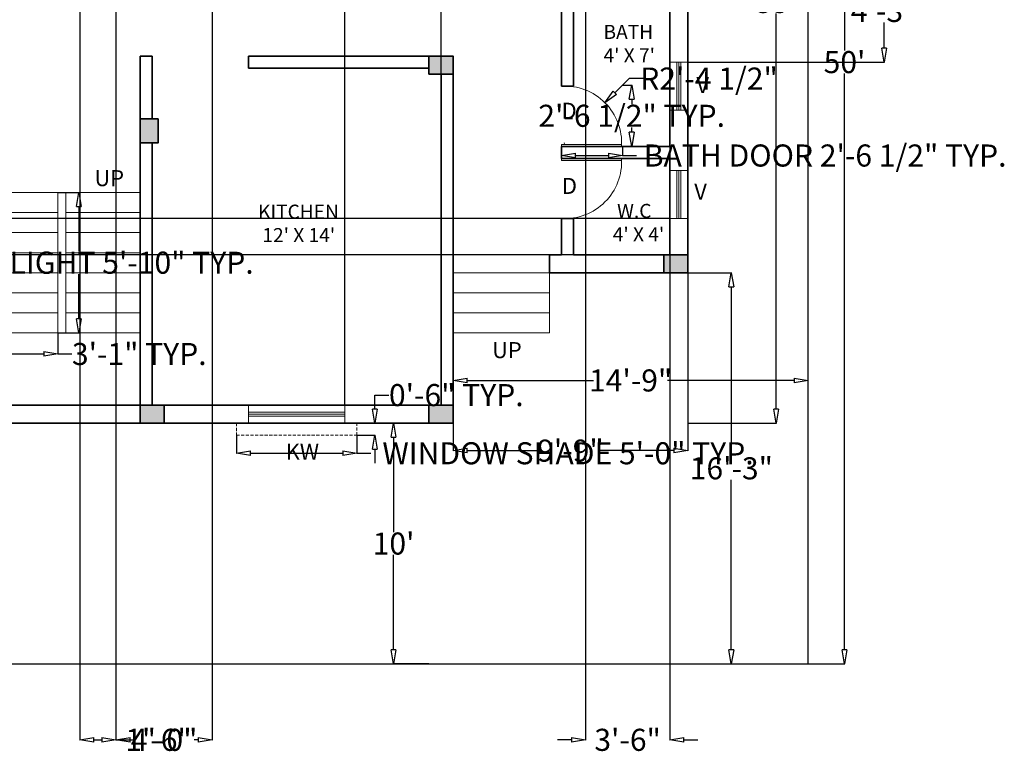
# Model space of a CAD drawing. Units: inches. Extents: x 668 to 1552, y 994 to 1684.
# Tile 3 of 4: x 1061 to 1552, y 994 to 1360. Entities that reach past the tile are written whole.
import ezdxf

# ---------------------------------------------------------------- set-up
doc = ezdxf.new("R2010")
doc.units = ezdxf.units.IN
doc.header["$LTSCALE"] = 2.5
doc.header["$MEASUREMENT"] = 0
doc.linetypes.add('HIDDEN', pattern=[0.375, 0.25, -0.125])
for name, color, linetype, lineweight, true_color in [('A-ANNO-DIMS', 175, 'Continuous', 13, 0x4554a5), ('A-ANNO-TEXT', 52, 'Continuous', 18, 0xc8c92d), ('A-DOOR', 152, 'Continuous', 18, 0x2776bb), ('A-FLOR-STRS', 165, 'Continuous', 18, 0x5e67af)]:
    doc.layers.add(name, color=color, linetype=linetype, lineweight=lineweight, true_color=true_color)
for name, color, linetype, lineweight in [('A-AREA-IDEN', 2, 'Continuous', 18), ('A-COLS', 7, 'Continuous', 35), ('A-COLS-PATT', 1, 'Continuous', 13), ('A-GLAZ', 4, 'Continuous', 18), ('A-WALL', 7, 'Continuous', 35), ('C-PROP', 1, 'Continuous', 25), ('sajjas', 210, 'HIDDEN', 13)]:
    doc.layers.add(name, color=color, linetype=linetype, lineweight=lineweight)
doc.styles.get("Standard").update_dxf_attribs({"font": 'arial.ttf'})
doc.dimstyles.get("Standard").update_dxf_attribs({"dimtxt": 11, "dimasz": 7, "dimexe": 0.18, "dimexo": 0.0625, "dimgap": 0.09, "dimtad": 0, "dimtih": 1, "dimtoh": 1, "dimdec": 0, "dimzin": 0, "dimdsep": 46, "dimlunit": 3, "dimtxsty": 'Standard', "dimblk": 'CLOSEDBLANK', "dimcen": 0.09, "dimadec": 0, "dimazin": 0, "dimtfac": 1, "dimtdec": 0, "dimtofl": 0, "dimtmove": 0, "dimatfit": 3, "dimldrblk": 'CLOSEDBLANK', "dimfxl": 1, "dimtolj": 1, "dimtzin": 0, "dimarcsym": 0})

# ---------------------------------------------------------------- blocks, each defined once
blk = doc.blocks.new('_ClosedBlank')
at = {"color": 0, "linetype": 'ByBlock', "lineweight": -2}
for p, q in [((-1, 0.167), (0, 0)), ((-1, 0.167), (-1, -0.167)), ((0, 0), (-1, -0.167))]:
    blk.add_line(p, q, dxfattribs=at)
blk = doc.blocks.new('*D2')
at = {"layer": 'A-ANNO-DIMS', "color": 0, "lineweight": -2, "ltscale": 2.5, "transparency": 16777216}
for p, q in [((1454.43, 1639.35), (1472.67, 1639.35)), ((1472.49, 1632.35), (1472.49, 1345.06)), ((1472.49, 1046.35), (1472.49, 1333.64)), ((1454.43, 1039.35), (1472.67, 1039.35))]:
    blk.add_line(p, q, dxfattribs=at)
at = {"layer": 'Defpoints', "color": 0, "ltscale": 2.5, "transparency": 16777216}
for p in [(1454.36, 1639.35), (1454.36, 1039.35), (1472.49, 1039.35)]:
    blk.add_point(p, dxfattribs=at)
at = {"layer": 'A-ANNO-DIMS', "color": 0, "lineweight": -2, "ltscale": 2.5, "transparency": 16777216, "xscale": 7, "yscale": 7, "zscale": 7}
for p, rotation in [((1472.49, 1639.35), 90), ((1472.49, 1039.35), 270)]:
    blk.add_blockref('_ClosedBlank', p, dxfattribs=dict(at, rotation=rotation))
at = {"layer": 'A-ANNO-DIMS', "color": 0, "ltscale": 2.5, "transparency": 16777216, "insert": (1472.49, 1339.35), "char_height": 11, "attachment_point": 5}
blk.add_mtext("\\A1;50'", dxfattribs=at)
blk = doc.blocks.new('*D9')
at = {"layer": 'A-ANNO-DIMS', "color": 0, "lineweight": -2, "ltscale": 2.5, "transparency": 16777216}
for p, q in [((1394.43, 1579.35), (1438.61, 1579.35)), ((1438.43, 1572.35), (1438.43, 1375.06)), ((1438.43, 1166.35), (1438.43, 1363.64)), ((1394.43, 1159.35), (1438.61, 1159.35))]:
    blk.add_line(p, q, dxfattribs=at)
at = {"layer": 'Defpoints', "color": 0, "ltscale": 2.5, "transparency": 16777216}
for p in [(1394.36, 1579.35), (1394.36, 1159.35), (1438.43, 1159.35)]:
    blk.add_point(p, dxfattribs=at)
at = {"layer": 'A-ANNO-DIMS', "color": 0, "lineweight": -2, "ltscale": 2.5, "transparency": 16777216, "xscale": 7, "yscale": 7, "zscale": 7}
for p, rotation in [((1438.43, 1579.35), 90), ((1438.43, 1159.35), 270)]:
    blk.add_blockref('_ClosedBlank', p, dxfattribs=dict(at, rotation=rotation))
at = {"layer": 'A-ANNO-DIMS', "color": 0, "ltscale": 2.5, "transparency": 16777216, "insert": (1438.43, 1369.35), "char_height": 11, "attachment_point": 5}
blk.add_mtext("\\A1;35'", dxfattribs=at)
blk = doc.blocks.new('*D10')
at = {"layer": 'A-ANNO-DIMS', "color": 0, "lineweight": -2, "ltscale": 2.5, "transparency": 16777216}
for p, q in [((1394.43, 1234.35), (1416.24, 1234.35)), ((1416.06, 1227.35), (1416.06, 1142.56)), ((1416.06, 1046.35), (1416.06, 1131.14)), ((1394.43, 1039.35), (1416.24, 1039.35))]:
    blk.add_line(p, q, dxfattribs=at)
at = {"layer": 'Defpoints', "color": 0, "ltscale": 2.5, "transparency": 16777216}
for p in [(1394.36, 1234.35), (1394.36, 1039.35), (1416.06, 1039.35)]:
    blk.add_point(p, dxfattribs=at)
at = {"layer": 'A-ANNO-DIMS', "color": 0, "lineweight": -2, "ltscale": 2.5, "transparency": 16777216, "xscale": 7, "yscale": 7, "zscale": 7}
for p, rotation in [((1416.06, 1234.35), 90), ((1416.06, 1039.35), 270)]:
    blk.add_blockref('_ClosedBlank', p, dxfattribs=dict(at, rotation=rotation))
at = {"layer": 'A-ANNO-DIMS', "color": 0, "ltscale": 2.5, "transparency": 16777216, "insert": (1416.06, 1136.85), "char_height": 11, "attachment_point": 5}
blk.add_mtext('\\A1;16\'-3"', dxfattribs=at)
blk = doc.blocks.new('*D11')
at = {"layer": 'A-ANNO-DIMS', "color": 0, "lineweight": -2, "ltscale": 2.5, "transparency": 16777216}
for p, q in [((1277.36, 1234.29), (1277.36, 1145.5)), ((1394.36, 1234.29), (1394.36, 1145.5)), ((1284.36, 1145.68), (1321.15, 1145.68)), ((1387.36, 1145.68), (1350.57, 1145.68))]:
    blk.add_line(p, q, dxfattribs=at)
at = {"layer": 'Defpoints', "color": 0, "ltscale": 2.5, "transparency": 16777216}
for p in [(1277.36, 1234.35), (1394.36, 1234.35), (1277.36, 1145.68)]:
    blk.add_point(p, dxfattribs=at)
at = {"layer": 'A-ANNO-DIMS', "color": 0, "lineweight": -2, "ltscale": 2.5, "transparency": 16777216, "xscale": 7, "yscale": 7, "zscale": 7, "rotation": 180}
blk.add_blockref('_ClosedBlank', (1277.36, 1145.68), dxfattribs=at)
at = {"layer": 'A-ANNO-DIMS', "color": 0, "lineweight": -2, "ltscale": 2.5, "transparency": 16777216, "xscale": 7, "yscale": 7, "zscale": 7}
blk.add_blockref('_ClosedBlank', (1394.36, 1145.68), dxfattribs=at)
at = {"layer": 'A-ANNO-DIMS', "color": 0, "ltscale": 2.5, "transparency": 16777216, "insert": (1335.86, 1145.68), "char_height": 11, "attachment_point": 5}
blk.add_mtext('\\A1;9\'-9"', dxfattribs=at)
blk = doc.blocks.new('*D12')
at = {"layer": 'A-ANNO-DIMS', "color": 0, "lineweight": -2, "ltscale": 2.5, "transparency": 16777216}
for p, q in [((1265.3, 1159.35), (1247.53, 1159.35)), ((1247.71, 1152.35), (1247.71, 1105.06)), ((1247.71, 1046.35), (1247.71, 1093.64)), ((1265.3, 1039.35), (1247.53, 1039.35))]:
    blk.add_line(p, q, dxfattribs=at)
at = {"layer": 'Defpoints', "color": 0, "ltscale": 2.5, "transparency": 16777216}
for p in [(1265.36, 1159.35), (1247.71, 1039.35), (1265.36, 1039.35)]:
    blk.add_point(p, dxfattribs=at)
at = {"layer": 'A-ANNO-DIMS', "color": 0, "lineweight": -2, "ltscale": 2.5, "transparency": 16777216, "xscale": 7, "yscale": 7, "zscale": 7}
for p, rotation in [((1247.71, 1159.35), 90), ((1247.71, 1039.35), 270)]:
    blk.add_blockref('_ClosedBlank', p, dxfattribs=dict(at, rotation=rotation))
at = {"layer": 'A-ANNO-DIMS', "color": 0, "ltscale": 2.5, "transparency": 16777216, "insert": (1247.71, 1099.35), "char_height": 11, "attachment_point": 5}
blk.add_mtext("\\A1;10'", dxfattribs=at)
blk = doc.blocks.new('*D13')
at = {"layer": 'A-ANNO-DIMS', "color": 0, "lineweight": -2, "ltscale": 2.5, "transparency": 16777216}
for p, q in [((1277.36, 1168.41), (1277.36, 1180.83)), ((1284.36, 1180.65), (1347.4, 1180.65)), ((1447.36, 1180.65), (1384.33, 1180.65)), ((1454.36, 1168.41), (1454.36, 1180.83))]:
    blk.add_line(p, q, dxfattribs=at)
at = {"layer": 'Defpoints', "color": 0, "ltscale": 2.5, "transparency": 16777216}
for p in [(1454.36, 1180.65), (1277.36, 1168.35), (1454.36, 1168.35)]:
    blk.add_point(p, dxfattribs=at)
at = {"layer": 'A-ANNO-DIMS', "color": 0, "lineweight": -2, "ltscale": 2.5, "transparency": 16777216, "xscale": 7, "yscale": 7, "zscale": 7, "rotation": 180}
blk.add_blockref('_ClosedBlank', (1277.36, 1180.65), dxfattribs=at)
at = {"layer": 'A-ANNO-DIMS', "color": 0, "lineweight": -2, "ltscale": 2.5, "transparency": 16777216, "xscale": 7, "yscale": 7, "zscale": 7}
blk.add_blockref('_ClosedBlank', (1454.36, 1180.65), dxfattribs=at)
at = {"layer": 'A-ANNO-DIMS', "color": 0, "ltscale": 2.5, "transparency": 16777216, "insert": (1365.86, 1180.65), "char_height": 11, "attachment_point": 5}
blk.add_mtext('\\A1;14\'-9"', dxfattribs=at)
blk = doc.blocks.new('WIN-48')
for p, q in [((0, 9), (48, 9)), ((0, 9), (0, 0)), ((48, 5.5), (0, 5.5)), ((48, 9), (48, 0)), ((48, 4.5), (0, 4.5)), ((48, 3.5), (0, 3.5)), ((0, 0), (48, 0))]:
    blk.add_line(p, q)
blk = doc.blocks.new('VENT-24')
for p, q in [((0, 9), (24, 9)), ((0, 0), (0, 9)), ((24, 5.5), (0.04, 5.5)), ((24, 9), (24, 0)), ((24, 0), (0, 0)), ((24, 4.5), (0.04, 4.5)), ((24, 3.5), (0.04, 3.5))]:
    blk.add_line(p, q)
blk = doc.blocks.new('SAJJA-60')
at = {"ltscale": 2.5}
blk.add_lwpolyline([(6, 6), (0, 6), (0, 0), (54, 0), (60, 0), (60, 6), (54, 6)], dxfattribs=at)
blk = doc.blocks.new('DOOR-BATH-30')
for p, q in [((0, 1), (30, 1)), ((0, 0), (30, 0))]:
    blk.add_line(p, q)
blk.add_arc((1.62, 1.62), 28.42, 356.7299, 93.2701)
blk = doc.blocks.new('STAIR-FLIGHT-37')
at = {"ltscale": 2.5}
for p, q in [((0, 70), (37, 70)), ((37, 0), (37, 70)), ((0, 60), (37, 60)), ((0, 50), (37, 50)), ((0, 40), (37, 40)), ((0, 30), (37, 30)), ((0, 20), (37, 20)), ((0, 10), (37, 10))]:
    blk.add_line(p, q, dxfattribs=at)
blk = doc.blocks.new('*D24')
at = {"layer": 'A-ANNO-DIMS', "color": 0, "lineweight": -2, "ltscale": 2.5, "transparency": 16777216}
for p, q in [((1169.36, 1153.29), (1169.36, 1144.17)), ((1229.36, 1153.29), (1229.36, 1144.17)), ((1176.36, 1144.35), (1222.36, 1144.35)), ((1229.36, 1144.35), (1236.36, 1144.35))]:
    blk.add_line(p, q, dxfattribs=at)
at = {"layer": 'Defpoints', "color": 0, "ltscale": 2.5, "transparency": 16777216}
for p in [(1169.36, 1153.35), (1229.36, 1153.35), (1229.36, 1144.35)]:
    blk.add_point(p, dxfattribs=at)
at = {"layer": 'A-ANNO-DIMS', "color": 0, "lineweight": -2, "ltscale": 2.5, "transparency": 16777216, "xscale": 7, "yscale": 7, "zscale": 7, "rotation": 180}
blk.add_blockref('_ClosedBlank', (1169.36, 1144.35), dxfattribs=at)
at = {"layer": 'A-ANNO-DIMS', "color": 0, "lineweight": -2, "ltscale": 2.5, "transparency": 16777216, "xscale": 7, "yscale": 7, "zscale": 7}
blk.add_blockref('_ClosedBlank', (1229.36, 1144.35), dxfattribs=at)
at = {"layer": 'A-ANNO-DIMS', "color": 0, "ltscale": 2.5, "transparency": 16777216, "insert": (1334.66, 1144.35), "char_height": 11, "attachment_point": 5}
blk.add_mtext('\\A1;WINDOW SHADE 5\'-0" TYP.', dxfattribs=at)
blk = doc.blocks.new('*D25')
at = {"layer": 'A-ANNO-DIMS', "color": 0, "lineweight": -2, "ltscale": 2.5, "transparency": 16777216}
for p, q in [((1238.36, 1166.35), (1238.36, 1173.35)), ((1238.36, 1173.35), (1245.36, 1173.35)), ((1229.43, 1159.35), (1238.54, 1159.35)), ((1229.43, 1153.35), (1238.54, 1153.35)), ((1238.36, 1146.35), (1238.36, 1139.35))]:
    blk.add_line(p, q, dxfattribs=at)
at = {"layer": 'Defpoints', "color": 0, "ltscale": 2.5, "transparency": 16777216}
for p in [(1229.36, 1159.35), (1238.36, 1159.35), (1229.36, 1153.35)]:
    blk.add_point(p, dxfattribs=at)
at = {"layer": 'A-ANNO-DIMS', "color": 0, "lineweight": -2, "ltscale": 2.5, "transparency": 16777216, "xscale": 7, "yscale": 7, "zscale": 7}
for p, rotation in [((1238.36, 1159.35), 270), ((1238.36, 1153.35), 90)]:
    blk.add_blockref('_ClosedBlank', p, dxfattribs=dict(at, rotation=rotation))
at = {"layer": 'A-ANNO-DIMS', "color": 0, "ltscale": 2.5, "transparency": 16777216, "insert": (1278.98, 1173.35), "char_height": 11, "attachment_point": 5}
blk.add_mtext('\\A1;0\'-6" TYP.', dxfattribs=at)
blk = doc.blocks.new('*D30')
at = {"layer": 'A-ANNO-DIMS', "color": 0, "lineweight": -2, "ltscale": 2.5, "transparency": 16777216}
for p, q in [((1331.36, 1297.29), (1331.36, 1292.6)), ((1361.82, 1297.29), (1361.82, 1292.6)), ((1338.36, 1292.78), (1354.82, 1292.78)), ((1361.82, 1292.78), (1368.82, 1292.78))]:
    blk.add_line(p, q, dxfattribs=at)
at = {"layer": 'Defpoints', "color": 0, "ltscale": 2.5, "transparency": 16777216}
for p in [(1331.36, 1297.35), (1361.82, 1297.35), (1361.82, 1292.78)]:
    blk.add_point(p, dxfattribs=at)
at = {"layer": 'A-ANNO-DIMS', "color": 0, "lineweight": -2, "ltscale": 2.5, "transparency": 16777216, "xscale": 7, "yscale": 7, "zscale": 7, "rotation": 180}
blk.add_blockref('_ClosedBlank', (1331.36, 1292.78), dxfattribs=at)
at = {"layer": 'A-ANNO-DIMS', "color": 0, "lineweight": -2, "ltscale": 2.5, "transparency": 16777216, "xscale": 7, "yscale": 7, "zscale": 7}
blk.add_blockref('_ClosedBlank', (1361.82, 1292.78), dxfattribs=at)
at = {"layer": 'A-ANNO-DIMS', "color": 0, "ltscale": 2.5, "transparency": 16777216, "insert": (1462.82, 1292.78), "char_height": 11, "attachment_point": 5}
blk.add_mtext('\\A1;BATH DOOR 2\'-6 1/2" TYP.', dxfattribs=at)
blk = doc.blocks.new('*D31')
at = {"layer": 'A-ANNO-DIMS', "color": 0, "lineweight": -2, "ltscale": 2.5, "transparency": 16777216}
for p, q in [((1361.89, 1327.81), (1366.57, 1327.81)), ((1366.39, 1320.81), (1366.39, 1318.36)), ((1366.39, 1304.35), (1366.39, 1306.8)), ((1361.89, 1297.35), (1366.57, 1297.35))]:
    blk.add_line(p, q, dxfattribs=at)
at = {"layer": 'Defpoints', "color": 0, "ltscale": 2.5, "transparency": 16777216}
for p in [(1361.82, 1327.81), (1366.39, 1327.81), (1361.82, 1297.35)]:
    blk.add_point(p, dxfattribs=at)
at = {"layer": 'A-ANNO-DIMS', "color": 0, "lineweight": -2, "ltscale": 2.5, "transparency": 16777216, "xscale": 7, "yscale": 7, "zscale": 7}
for p, rotation in [((1366.39, 1327.81), 90), ((1366.39, 1297.35), 270)]:
    blk.add_blockref('_ClosedBlank', p, dxfattribs=dict(at, rotation=rotation))
at = {"layer": 'A-ANNO-DIMS', "color": 0, "ltscale": 2.5, "transparency": 16777216, "insert": (1366.39, 1312.58), "char_height": 11, "attachment_point": 5}
blk.add_mtext('\\A1;2\'-6 1/2" TYP.', dxfattribs=at)
blk = doc.blocks.new('*D32')
at = {"layer": 'A-ANNO-DIMS', "color": 0, "lineweight": -2, "ltscale": 2.5, "transparency": 16777216}
for p, q in [((1080.43, 1274.35), (1091.04, 1274.35)), ((1090.86, 1267.35), (1090.86, 1245.13)), ((1090.86, 1211.35), (1090.86, 1233.57)), ((1080.43, 1204.35), (1091.04, 1204.35))]:
    blk.add_line(p, q, dxfattribs=at)
at = {"layer": 'Defpoints', "color": 0, "ltscale": 2.5, "transparency": 16777216}
for p in [(1080.36, 1274.35), (1090.86, 1274.35), (1080.36, 1204.35)]:
    blk.add_point(p, dxfattribs=at)
at = {"layer": 'A-ANNO-DIMS', "color": 0, "lineweight": -2, "ltscale": 2.5, "transparency": 16777216, "xscale": 7, "yscale": 7, "zscale": 7}
for p, rotation in [((1090.86, 1274.35), 90), ((1090.86, 1204.35), 270)]:
    blk.add_blockref('_ClosedBlank', p, dxfattribs=dict(at, rotation=rotation))
at = {"layer": 'A-ANNO-DIMS', "color": 0, "ltscale": 2.5, "transparency": 16777216, "insert": (1090.86, 1239.35), "char_height": 11, "attachment_point": 5}
blk.add_mtext('\\A1;STAIR FLIGHT 5\'-10" TYP.', dxfattribs=at)
blk = doc.blocks.new('*D33')
at = {"layer": 'A-ANNO-DIMS', "color": 0, "lineweight": -2, "ltscale": 2.5, "transparency": 16777216}
for p, q in [((1043.36, 1204.29), (1043.36, 1193.67)), ((1080.36, 1204.29), (1080.36, 1193.67)), ((1050.36, 1193.85), (1073.36, 1193.85)), ((1080.36, 1193.85), (1087.36, 1193.85))]:
    blk.add_line(p, q, dxfattribs=at)
at = {"layer": 'Defpoints', "color": 0, "ltscale": 2.5, "transparency": 16777216}
for p in [(1043.36, 1204.35), (1080.36, 1204.35), (1080.36, 1193.85)]:
    blk.add_point(p, dxfattribs=at)
at = {"layer": 'A-ANNO-DIMS', "color": 0, "lineweight": -2, "ltscale": 2.5, "transparency": 16777216, "xscale": 7, "yscale": 7, "zscale": 7, "rotation": 180}
blk.add_blockref('_ClosedBlank', (1043.36, 1193.85), dxfattribs=at)
at = {"layer": 'A-ANNO-DIMS', "color": 0, "lineweight": -2, "ltscale": 2.5, "transparency": 16777216, "xscale": 7, "yscale": 7, "zscale": 7}
blk.add_blockref('_ClosedBlank', (1080.36, 1193.85), dxfattribs=at)
at = {"layer": 'A-ANNO-DIMS', "color": 0, "ltscale": 2.5, "transparency": 16777216, "insert": (1120.97, 1193.85), "char_height": 11, "attachment_point": 5}
blk.add_mtext('\\A1;3\'-1" TYP.', dxfattribs=at)
blk = doc.blocks.new('*D39')
at = {"layer": 'A-ANNO-DIMS', "color": 0, "lineweight": -2, "ltscale": 2.5, "transparency": 16777216}
for p, q in [((1091.36, 1570.29), (1091.36, 1001.32)), ((1109.36, 1570.29), (1109.36, 1001.32)), ((1098.36, 1001.5), (1102.36, 1001.5)), ((1109.36, 1001.5), (1116.36, 1001.5))]:
    blk.add_line(p, q, dxfattribs=at)
at = {"layer": 'Defpoints', "color": 0, "ltscale": 2.5, "transparency": 16777216}
for p in [(1091.36, 1570.35), (1109.36, 1570.35), (1109.36, 1001.5)]:
    blk.add_point(p, dxfattribs=at)
at = {"layer": 'A-ANNO-DIMS', "color": 0, "lineweight": -2, "ltscale": 2.5, "transparency": 16777216, "xscale": 7, "yscale": 7, "zscale": 7, "rotation": 180}
blk.add_blockref('_ClosedBlank', (1091.36, 1001.5), dxfattribs=at)
at = {"layer": 'A-ANNO-DIMS', "color": 0, "lineweight": -2, "ltscale": 2.5, "transparency": 16777216, "xscale": 7, "yscale": 7, "zscale": 7}
blk.add_blockref('_ClosedBlank', (1109.36, 1001.5), dxfattribs=at)
at = {"layer": 'A-ANNO-DIMS', "color": 0, "ltscale": 2.5, "transparency": 16777216, "insert": (1130.56, 1001.5), "char_height": 11, "attachment_point": 5}
blk.add_mtext('\\A1;1\'-6"', dxfattribs=at)
blk = doc.blocks.new('*D40')
at = {"layer": 'A-ANNO-DIMS', "color": 0, "lineweight": -2, "ltscale": 2.5, "transparency": 16777216}
for p, q in [((1109.36, 1570.29), (1109.36, 1001.32)), ((1157.36, 1570.29), (1157.36, 1001.32)), ((1116.36, 1001.5), (1118.43, 1001.5)), ((1150.36, 1001.5), (1148.29, 1001.5))]:
    blk.add_line(p, q, dxfattribs=at)
at = {"layer": 'Defpoints', "color": 0, "ltscale": 2.5, "transparency": 16777216}
for p in [(1109.36, 1570.35), (1157.36, 1570.35), (1157.36, 1001.5)]:
    blk.add_point(p, dxfattribs=at)
at = {"layer": 'A-ANNO-DIMS', "color": 0, "lineweight": -2, "ltscale": 2.5, "transparency": 16777216, "xscale": 7, "yscale": 7, "zscale": 7, "rotation": 180}
blk.add_blockref('_ClosedBlank', (1109.36, 1001.5), dxfattribs=at)
at = {"layer": 'A-ANNO-DIMS', "color": 0, "lineweight": -2, "ltscale": 2.5, "transparency": 16777216, "xscale": 7, "yscale": 7, "zscale": 7}
blk.add_blockref('_ClosedBlank', (1157.36, 1001.5), dxfattribs=at)
at = {"layer": 'A-ANNO-DIMS', "color": 0, "ltscale": 2.5, "transparency": 16777216, "insert": (1133.36, 1001.5), "char_height": 11, "attachment_point": 5}
blk.add_mtext('\\A1;4\'-0"', dxfattribs=at)
blk = doc.blocks.new('*D41')
at = {"layer": 'A-ANNO-DIMS', "color": 0, "lineweight": -2, "ltscale": 2.5, "transparency": 16777216}
for p, q in [((1343.362549, 1570.287512), (1343.362549, 1001.320012)), ((1385.362549, 1570.287512), (1385.362549, 1001.320012)), ((1336.362549, 1001.500012), (1329.362549, 1001.500012)), ((1392.362549, 1001.500012), (1399.362549, 1001.500012))]:
    blk.add_line(p, q, dxfattribs=at)
at = {"layer": 'Defpoints', "color": 0, "ltscale": 2.5, "transparency": 16777216}
for p in [(1343.362549, 1570.350012), (1385.362549, 1570.350012), (1385.362549, 1001.500012)]:
    blk.add_point(p, dxfattribs=at)
at = {"layer": 'A-ANNO-DIMS', "color": 0, "lineweight": -2, "ltscale": 2.5, "transparency": 16777216, "xscale": 7, "yscale": 7, "zscale": 7}
blk.add_blockref('_ClosedBlank', (1343.362549, 1001.500012), dxfattribs=at)
at = {"layer": 'A-ANNO-DIMS', "color": 0, "lineweight": -2, "ltscale": 2.5, "transparency": 16777216, "xscale": 7, "yscale": 7, "zscale": 7, "rotation": 180}
blk.add_blockref('_ClosedBlank', (1385.362549, 1001.500012), dxfattribs=at)
at = {"layer": 'A-ANNO-DIMS', "color": 0, "ltscale": 2.5, "transparency": 16777216, "insert": (1364.362549, 1001.500012), "char_height": 11, "attachment_point": 5}
blk.add_mtext('\\A1;3\'-6"', dxfattribs=at)
blk = doc.blocks.new('*D49')
at = {"layer": 'A-ANNO-DIMS', "color": 0, "lineweight": -2, "ltscale": 2.5, "transparency": 16777216}
for p, q in [((1223.36, 1168.41), (1223.36, 1677.38)), ((1230.36, 1677.2), (1232.43, 1677.2)), ((1264.36, 1677.2), (1262.29, 1677.2)), ((1271.36, 1168.41), (1271.36, 1677.38))]:
    blk.add_line(p, q, dxfattribs=at)
at = {"layer": 'Defpoints', "color": 0, "ltscale": 2.5, "transparency": 16777216}
for p in [(1271.36, 1677.2), (1223.36, 1168.35), (1271.36, 1168.35)]:
    blk.add_point(p, dxfattribs=at)
at = {"layer": 'A-ANNO-DIMS', "color": 0, "lineweight": -2, "ltscale": 2.5, "transparency": 16777216, "xscale": 7, "yscale": 7, "zscale": 7, "rotation": 180}
blk.add_blockref('_ClosedBlank', (1223.36, 1677.2), dxfattribs=at)
at = {"layer": 'A-ANNO-DIMS', "color": 0, "lineweight": -2, "ltscale": 2.5, "transparency": 16777216, "xscale": 7, "yscale": 7, "zscale": 7}
blk.add_blockref('_ClosedBlank', (1271.36, 1677.2), dxfattribs=at)
at = {"layer": 'A-ANNO-DIMS', "color": 0, "ltscale": 2.5, "transparency": 16777216, "insert": (1247.36, 1677.2), "char_height": 11, "attachment_point": 5}
blk.add_mtext('\\A1;4\'-0"', dxfattribs=at)
blk = doc.blocks.new('*D50')
at = {"layer": 'A-ANNO-DIMS', "color": 0, "lineweight": -2, "ltscale": 2.5, "transparency": 16777216}
for p, q in [((1394.43, 1390.35), (1492.39, 1390.35)), ((1492.21, 1383.35), (1492.21, 1370.56)), ((1492.21, 1346.35), (1492.21, 1359.14)), ((1394.43, 1339.35), (1492.39, 1339.35))]:
    blk.add_line(p, q, dxfattribs=at)
at = {"layer": 'Defpoints', "color": 0, "ltscale": 2.5, "transparency": 16777216}
for p in [(1394.36, 1390.35), (1394.36, 1339.35), (1492.21, 1339.35)]:
    blk.add_point(p, dxfattribs=at)
at = {"layer": 'A-ANNO-DIMS', "color": 0, "lineweight": -2, "ltscale": 2.5, "transparency": 16777216, "xscale": 7, "yscale": 7, "zscale": 7}
for p, rotation in [((1492.21, 1390.35), 90), ((1492.21, 1339.35), 270)]:
    blk.add_blockref('_ClosedBlank', p, dxfattribs=dict(at, rotation=rotation))
at = {"layer": 'A-ANNO-DIMS', "color": 0, "ltscale": 2.5, "transparency": 16777216, "insert": (1492.21, 1364.85), "char_height": 11, "attachment_point": 5}
blk.add_mtext('\\A1;4\'-3"', dxfattribs=at)
blk = doc.blocks.new('*D51')
at = {"layer": 'A-ANNO-DIMS', "color": 0, "lineweight": -2, "ltscale": 2.5, "transparency": 16777216}
for p, q in [((696.51, 1261.35), (696.51, 1268.35)), ((696.51, 1268.35), (703.51, 1268.35)), ((1385.3, 1261.35), (696.33, 1261.35)), ((696.51, 1250.35), (696.51, 1254.35)), ((1385.3, 1243.35), (696.33, 1243.35))]:
    blk.add_line(p, q, dxfattribs=at)
at = {"layer": 'Defpoints', "color": 0, "ltscale": 2.5, "transparency": 16777216}
for p in [(696.51, 1261.35), (1385.36, 1261.35), (1385.36, 1243.35)]:
    blk.add_point(p, dxfattribs=at)
at = {"layer": 'A-ANNO-DIMS', "color": 0, "lineweight": -2, "ltscale": 2.5, "transparency": 16777216, "xscale": 7, "yscale": 7, "zscale": 7}
for p, rotation in [((696.51, 1261.35), 90), ((696.51, 1243.35), 270)]:
    blk.add_blockref('_ClosedBlank', p, dxfattribs=dict(at, rotation=rotation))
at = {"layer": 'A-ANNO-DIMS', "color": 0, "ltscale": 2.5, "transparency": 16777216, "insert": (717.71, 1268.35), "char_height": 11, "attachment_point": 5}
blk.add_mtext('\\A1;1\'-6"', dxfattribs=at)
blk = doc.blocks.new('*D58')
at = {"layer": 'A-ANNO-DIMS', "color": 0, "lineweight": -2, "ltscale": 2.5, "transparency": 16777216}
for p, q in [((1365.14, 1331.13), (1358.03, 1324.02)), ((1372.14, 1331.13), (1365.14, 1331.13)), ((1332.89, 1298.97), (1333.07, 1298.97)), ((1332.98, 1298.88), (1332.98, 1299.06))]:
    blk.add_line(p, q, dxfattribs=at)
at = {"layer": 'Defpoints', "color": 0, "ltscale": 2.5, "transparency": 16777216}
for p in [(1353.08, 1319.07), (1332.98, 1298.97)]:
    blk.add_point(p, dxfattribs=at)
at = {"layer": 'A-ANNO-DIMS', "color": 0, "lineweight": -2, "ltscale": 2.5, "transparency": 16777216, "xscale": 7, "yscale": 7, "zscale": 7, "rotation": 225.0007653918236}
blk.add_blockref('_ClosedBlank', (1353.08, 1319.07), dxfattribs=at)
at = {"layer": 'A-ANNO-DIMS', "color": 0, "ltscale": 2.5, "transparency": 16777216, "insert": (1404.93, 1331.13), "char_height": 11, "attachment_point": 5}
blk.add_mtext('\\A1;R2\'-4 1/2"', dxfattribs=at)

msp = doc.modelspace()

# ---------------------------------------------------------------- hatches: boundary and pattern name
at = {"layer": 'A-COLS-PATT'}
h = msp.add_hatch(color=256, dxfattribs=at)
h.dxf.hatch_style = 1
h.paths.add_polyline_path([(803.36, 1390.35), (794.36, 1390.35), (794.36, 1378.35), (803.36, 1378.35)])
h.paths.add_polyline_path([(1117.36, 1393.35), (1108.36, 1393.35), (1108.36, 1381.35), (1117.36, 1381.35)])
h.paths.add_polyline_path([(1255.36, 1390.35), (1243.36, 1390.35), (1243.36, 1381.35), (1255.36, 1381.35)])
h.paths.add_polyline_path([(1394.36, 1390.35), (1382.36, 1390.35), (1382.36, 1381.35), (1394.36, 1381.35)])
h.paths.add_polyline_path([(1394.36, 1579.35), (1385.36, 1579.35), (1385.36, 1567.35), (1394.36, 1567.35)])
h.paths.add_polyline_path([(1253.36, 1579.35), (1241.36, 1579.35), (1241.36, 1570.35), (1253.36, 1570.35)])
h.paths.add_polyline_path([(1115.36, 1579.35), (1103.36, 1579.35), (1103.36, 1570.35), (1115.36, 1570.35)])
h.paths.add_polyline_path([(923.36, 1579.35), (914.36, 1579.35), (914.36, 1567.35), (923.36, 1567.35)])
h.paths.add_polyline_path([(926.36, 1390.35), (914.36, 1390.35), (914.36, 1381.35), (926.36, 1381.35)])
h.paths.add_polyline_path([(1394.36, 1243.35), (1382.36, 1243.35), (1382.36, 1234.35), (1394.36, 1234.35)])
h.paths.add_polyline_path([(1277.36, 1342.35), (1265.36, 1342.35), (1265.36, 1333.35), (1277.36, 1333.35)])
h.paths.add_polyline_path([(1130.36, 1311.02), (1121.36, 1311.02), (1121.36, 1299.02), (1130.36, 1299.02)])
h.paths.add_polyline_path([(1043.36, 1311.02), (1034.36, 1311.02), (1034.36, 1299.02), (1043.36, 1299.02)])
h.paths.add_polyline_path([(803.36, 1171.35), (794.36, 1171.35), (794.36, 1159.35), (803.36, 1159.35)])
h.paths.add_polyline_path([(1046.36, 1168.35), (1034.36, 1168.35), (1034.36, 1159.35), (1046.36, 1159.35)])
h.paths.add_polyline_path([(1133.36, 1168.35), (1121.36, 1168.35), (1121.36, 1159.35), (1133.36, 1159.35)])
h.paths.add_polyline_path([(1277.36, 1168.35), (1265.36, 1168.35), (1265.36, 1159.35), (1277.36, 1159.35)])

# ---------------------------------------------------------------- linework, layer by layer
at = {"layer": 'A-COLS'}
for points in [[(1277.36, 1333.35), (1277.36, 1342.35), (1265.36, 1342.35), (1265.36, 1333.35)], [(1121.36, 1299.02), (1130.36, 1299.02), (1130.36, 1311.02), (1121.36, 1311.02)], [(1394.36, 1234.35), (1394.36, 1243.35), (1382.36, 1243.35), (1382.36, 1234.35)], [(1133.36, 1159.35), (1133.36, 1168.35), (1121.36, 1168.35), (1121.36, 1159.35)], [(1277.36, 1159.35), (1277.36, 1168.35), (1265.36, 1168.35), (1265.36, 1159.35)]]:
    msp.add_lwpolyline(points, close=True, dxfattribs=at)
at = {"layer": 'A-DOOR'}
for p, q in [((1331.36, 1298.35), (1331.36, 1297.06)), ((1331.36, 1290.35), (1331.36, 1291.35))]:
    msp.add_line(p, q, dxfattribs=at)
at = {"layer": 'A-FLOR-STRS', "ltscale": 2.5}
for p, q in [((1325.36, 1234.35), (1277.36, 1234.35)), ((1325.36, 1204.35), (1325.36, 1234.35)), ((1325.36, 1224.35), (1277.36, 1224.35)), ((1325.36, 1214.35), (1277.36, 1214.35)), ((1043.36, 1204.35), (1121.36, 1204.35)), ((1325.36, 1204.35), (1277.36, 1204.35))]:
    msp.add_line(p, q, dxfattribs=at)
at = {"layer": 'A-GLAZ'}
for p, q in [((1385.36, 1339.35), (1394.36, 1339.35)), ((1385.36, 1261.35), (1394.36, 1261.35))]:
    msp.add_line(p, q, dxfattribs=at)
at = {"layer": 'A-WALL'}
for p, q in [((1394.36, 1234.35), (1394.36, 1579.35)), ((1331.36, 1327.35), (1331.36, 1381.35)), ((1337.36, 1327.35), (1337.36, 1381.35)), ((1385.36, 1297.35), (1385.36, 1381.35)), ((1121.36, 1342.35), (1121.36, 1168.35)), ((1121.36, 1342.35), (1127.36, 1342.35)), ((1127.36, 1336.35), (1127.36, 1342.35)), ((1175.36, 1336.35), (1175.36, 1342.35)), ((1175.36, 1342.35), (1277.36, 1342.35)), ((1277.36, 1342.35), (1277.36, 1159.35)), ((1127.36, 1336.35), (1127.36, 1311.02)), ((1175.36, 1336.35), (1265.36, 1336.35)), ((1271.36, 1333.35), (1271.36, 1168.35)), ((1337.36, 1327.35), (1331.36, 1327.35)), ((1127.36, 1299.02), (1127.36, 1168.35)), ((1337.36, 1297.35), (1331.36, 1297.35)), ((1331.36, 1291.35), (1331.36, 1297.35)), ((1385.36, 1297.35), (1337.36, 1297.35)), ((1337.36, 1291.35), (1331.36, 1291.35)), ((1337.36, 1291.35), (1331.36, 1291.35)), ((1385.36, 1291.35), (1337.36, 1291.35)), ((1385.36, 1243.35), (1385.36, 1291.35)), ((1331.36, 1243.35), (1331.36, 1261.35)), ((1337.36, 1261.35), (1331.36, 1261.35)), ((1337.36, 1261.35), (1331.36, 1261.35)), ((1337.36, 1243.35), (1337.36, 1261.35)), ((1325.36, 1240.35), (1325.36, 1243.35)), ((1325.36, 1243.35), (1331.36, 1243.35)), ((1385.36, 1243.35), (1337.36, 1243.35)), ((1325.36, 1234.35), (1325.36, 1240.35)), ((1331.36, 1234.35), (1325.36, 1234.35)), ((1394.36, 1234.35), (1331.36, 1234.35)), ((1043.36, 1168.35), (1121.36, 1168.35)), ((1127.36, 1168.35), (1271.36, 1168.35)), ((1034.36, 1159.35), (1277.36, 1159.35))]:
    msp.add_line(p, q, dxfattribs=at)
at = {"layer": 'C-PROP', "ltscale": 2.5}
for p, q in [((1454.36, 1039.35), (1454.36, 1639.35)), ((734.36, 1039.35), (1454.36, 1039.35))]:
    msp.add_line(p, q, dxfattribs=at)

# ---------------------------------------------------------------- block references
at = {"layer": 'A-DOOR'}
msp.add_blockref('DOOR-BATH-30', (1331.36, 1297.35), dxfattribs=at)
at = {"layer": 'A-DOOR', "extrusion": (0, 0, -1), "zscale": -1, "rotation": 180}
msp.add_blockref('DOOR-BATH-30', (-1331.36, 1291.35), dxfattribs=at)
at = {"layer": 'A-FLOR-STRS'}
msp.add_blockref('STAIR-FLIGHT-37', (1043.36, 1204.35), dxfattribs=at)
at = {"layer": 'A-FLOR-STRS', "extrusion": (0, 0, -1), "zscale": -1}
msp.add_blockref('STAIR-FLIGHT-37', (-1121.36, 1204.35), dxfattribs=at)
at = {"layer": 'A-GLAZ'}
for name, p, rotation in [('VENT-24', (1394.36, 1315.35), 90.00000000000072), ('VENT-24', (1394.36, 1261.35), 90.00000000000072), ('WIN-48', (1223.36, 1168.35), 180)]:
    msp.add_blockref(name, p, dxfattribs=dict(at, rotation=rotation))
at = {"layer": 'sajjas'}
msp.add_blockref('SAJJA-60', (1169.36, 1153.35), dxfattribs=at)

# ---------------------------------------------------------------- texts
at = {"layer": 'A-ANNO-TEXT', "ltscale": 2.5, "char_height": 8, "attachment_point": 1}
for s, insert in [('V', (1398.64, 1331.88)), ('D', (1331.47, 1319.09)), ('UP', (1098.62, 1285.5)), ('D', (1331.63, 1281.63)), ('V', (1397.58, 1278.76)), ('UP', (1296.83, 1199.77)), ('KW', (1193.93, 1149.09))]:
    msp.add_mtext_dynamic_manual_height_columns(s, width=96.0512, gutter_width=1, heights=[0], dxfattribs=dict(at, insert=insert))
at = {"layer": 'A-AREA-IDEN', "ltscale": 2.5, "char_height": 7, "attachment_point": 1}
for s, width, insert in [("BATH\\P4' X 7'", 46.3724, (1352.34, 1357.89)), ("KITCHEN\\P 12' X 14'", 64.041, (1180.19, 1268.28)), (" W.C\\P4' X 4'", 47.3322, (1356.97, 1268.67))]:
    msp.add_mtext_dynamic_manual_height_columns(s, width=width, gutter_width=1, heights=[0], dxfattribs=dict(at, insert=insert))

# ---------------------------------------------------------------- dimensions: what is measured, and where the dimension line sits
at = {"layer": 'A-ANNO-DIMS', "ltscale": 2.5}
for base, p1, p2, override, picture, middle in [((1271.36, 1677.2), (1223.36, 1168.35), (1271.36, 1168.35), {"dimdec": 1, "dimlfac": 1, "dimrnd": 0, "dimzin": 1, "dimdsep": 46, "dimlunit": 4, "dimfrac": 2}, '*D49', (1247.36, 1677.2)), ((1109.36, 1001.5), (1091.36, 1570.35), (1109.36, 1570.35), {"dimdec": 1, "dimlfac": 1, "dimrnd": 0, "dimzin": 1, "dimdsep": 46, "dimlunit": 4, "dimfrac": 2}, '*D39', (1130.56, 1001.5)), ((1157.36, 1001.5), (1109.36, 1570.35), (1157.36, 1570.35), {"dimdec": 1, "dimlfac": 1, "dimrnd": 0, "dimzin": 1, "dimdsep": 46, "dimlunit": 4, "dimfrac": 2}, '*D40', (1133.36, 1001.5)), ((1385.36, 1001.5), (1343.36, 1570.35), (1385.36, 1570.35), {"dimdec": 1, "dimlfac": 1, "dimrnd": 0, "dimzin": 1, "dimdsep": 46, "dimlunit": 4, "dimfrac": 2}, '*D41', (1364.36, 1001.5)), ((1277.36, 1145.68), (1394.36, 1234.35), (1277.36, 1234.35), {"dimclrd": 0, "dimclre": 0, "dimclrt": 0}, '*D11', (1335.86, 1145.68)), ((1454.36, 1180.65), (1277.36, 1168.35), (1454.36, 1168.35), {"dimclrd": 0, "dimclre": 0, "dimclrt": 0}, '*D13', (1365.86, 1180.65))]:
    dim = msp.add_linear_dim(base=base, p1=p1, p2=p2, dimstyle='Standard', override=override, dxfattribs=at)
    dim.commit()
    dim.dimension.update_dxf_attribs({"geometry": picture, "text_midpoint": middle})
for base, p1, p2, override, picture, middle in [((1472.49, 1039.35), (1454.36, 1639.35), (1454.36, 1039.35), {"dimclrd": 0, "dimclre": 0, "dimclrt": 0}, '*D2', (1472.49, 1339.35)), ((1438.43, 1159.35), (1394.36, 1579.35), (1394.36, 1159.35), {"dimclrd": 0, "dimclre": 0, "dimclrt": 0}, '*D9', (1438.43, 1369.35)), ((1492.21, 1339.35), (1394.36, 1390.35), (1394.36, 1339.35), {"dimdec": 1, "dimlfac": 1, "dimrnd": 0, "dimzin": 1, "dimdsep": 46, "dimlunit": 4, "dimfrac": 2}, '*D50', (1492.21, 1364.85)), ((696.51, 1261.35), (1385.36, 1243.35), (1385.36, 1261.35), {"dimdec": 1, "dimlfac": 1, "dimrnd": 0, "dimzin": 1, "dimdsep": 46, "dimlunit": 4, "dimfrac": 2}, '*D51', (717.71, 1268.35)), ((1416.06, 1039.35), (1394.36, 1234.35), (1394.36, 1039.35), {"dimclrd": 0, "dimclre": 0, "dimclrt": 0}, '*D10', (1416.06, 1136.85)), ((1247.71, 1039.35), (1265.36, 1159.35), (1265.36, 1039.35), {"dimclrd": 0, "dimclre": 0, "dimclrt": 0}, '*D12', (1247.71, 1099.35))]:
    dim = msp.add_linear_dim(base=base, p1=p1, p2=p2, angle=90, dimstyle='Standard', override=override, dxfattribs=at)
    dim.commit()
    dim.dimension.update_dxf_attribs({"geometry": picture, "text_midpoint": middle})
dim = msp.add_radius_dim(center=(1332.98, 1298.97), mpoint=(1353.08, 1319.07), dimstyle='Standard', override={"dimdec": 1, "dimlfac": 1, "dimrnd": 0, "dimzin": 1, "dimdsep": 46, "dimlunit": 4, "dimfrac": 2}, dxfattribs=at)
dim.commit()
dim.dimension.update_dxf_attribs({"geometry": '*D58', "text_midpoint": (1404.93, 1331.13), "dimtype": 164})
for base, p1, p2, text, picture, middle in [((1366.39, 1327.81), (1361.82, 1297.35), (1361.82, 1327.81), '<> TYP.', '*D31', (1366.39, 1312.58)), ((1090.86, 1274.35), (1080.36, 1204.35), (1080.36, 1274.35), 'STAIR FLIGHT <> TYP.', '*D32', (1090.86, 1239.35)), ((1238.36, 1159.35), (1229.36, 1153.35), (1229.36, 1159.35), '<> TYP.', '*D25', (1278.98, 1173.35))]:
    dim = msp.add_linear_dim(base=base, p1=p1, p2=p2, angle=90, text=text, dimstyle='Standard', override={"dimdec": 1, "dimlfac": 1, "dimrnd": 0, "dimzin": 1, "dimdsep": 46, "dimlunit": 4, "dimfrac": 2}, dxfattribs=at)
    dim.commit()
    dim.dimension.update_dxf_attribs({"geometry": picture, "text_midpoint": middle})
for base, p1, p2, text, picture, middle in [((1361.82, 1292.78), (1331.36, 1297.35), (1361.82, 1297.35), 'BATH DOOR <> TYP.', '*D30', (1462.82, 1292.78)), ((1080.36, 1193.85), (1043.36, 1204.35), (1080.36, 1204.35), '<> TYP.', '*D33', (1120.97, 1193.85)), ((1229.36, 1144.35), (1169.36, 1153.35), (1229.36, 1153.35), 'WINDOW SHADE <> TYP.', '*D24', (1334.66, 1144.35))]:
    dim = msp.add_linear_dim(base=base, p1=p1, p2=p2, text=text, dimstyle='Standard', override={"dimdec": 1, "dimlfac": 1, "dimrnd": 0, "dimzin": 1, "dimdsep": 46, "dimlunit": 4, "dimfrac": 2}, dxfattribs=at)
    dim.commit()
    dim.dimension.update_dxf_attribs({"geometry": picture, "text_midpoint": middle})

doc.saveas('drawing.dxf')
